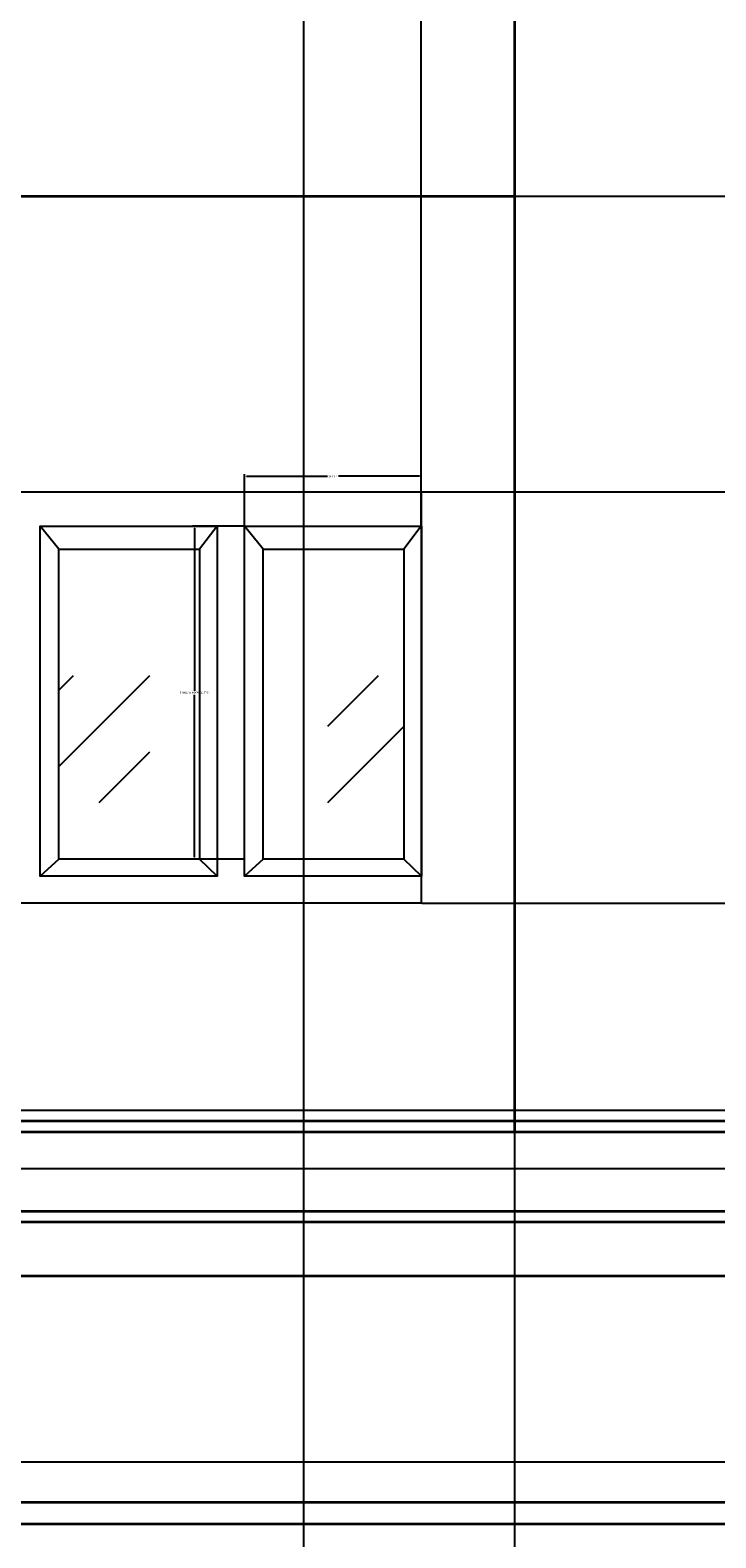
# Model space of a CAD drawing. Units: inches. Extents: x 93 to 565, y 123 to 656.
# Tile 10 of 18: x 393 to 456, y 324 to 463. Entities that reach past the tile are written whole.
import ezdxf

# ---------------------------------------------------------------- set-up
doc = ezdxf.new("R2010")
doc.units = ezdxf.units.IN
doc.header["$MEASUREMENT"] = 0
for name, color, linetype, lineweight in [('A-ANNO-DIMS', 2, 'Continuous', 18), ('A-ELEV', 7, 'Continuous', 35), ('A-GLAZ', 4, 'Continuous', 25)]:
    doc.layers.add(name, color=color, linetype=linetype, lineweight=lineweight)
doc.styles.get("Standard").update_dxf_attribs({"font": 'arial.ttf'})
doc.dimstyles.get("Standard").update_dxf_attribs({"dimtxt": 0.18, "dimasz": 0.18, "dimexe": 0.18, "dimexo": 0.0625, "dimgap": 0.09, "dimtad": 0, "dimtih": 1, "dimtoh": 1, "dimdec": 4, "dimzin": 0, "dimdsep": 46, "dimtxsty": 'Standard', "dimcen": 0.09, "dimadec": 0, "dimazin": 0, "dimtfac": 1, "dimtdec": 4, "dimtofl": 0, "dimtmove": 0, "dimatfit": 3, "dimfxl": 1, "dimtolj": 1, "dimtzin": 0, "dimarcsym": 0})

# ---------------------------------------------------------------- blocks, each defined once
blk = doc.blocks.new('WIN-CASEMENT-SMALL')
blk.add_lwpolyline([(1.71, 28.48), (0, 30.59), (16.23, 30.59), (14.61, 28.48)])
blk.add_lwpolyline([(1.71, 28.48), (14.61, 28.48), (14.61, 0), (1.71, 0)], close=True)
blk = doc.blocks.new('*D16')
at = {"layer": 'A-ANNO-DIMS', "color": 0, "lineweight": -2, "transparency": 16777216}
for p, q in [((412.34, 417.42), (407.63, 417.42)), ((407.81, 417.24), (407.81, 402.31)), ((407.81, 387.01), (407.81, 401.94)), ((412.34, 386.83), (407.63, 386.83))]:
    blk.add_line(p, q, dxfattribs=at)
at = {"layer": 'A-ANNO-DIMS', "color": 0, "transparency": 16777216}
for points in [[(407.78, 417.24), (407.84, 417.24), (407.81, 417.42)], [(407.78, 387.01), (407.84, 387.01), (407.81, 386.83)]]:
    blk.add_solid(points, dxfattribs=at)
at = {"layer": 'Defpoints', "color": 0, "transparency": 16777216}
for p in [(407.81, 417.42), (412.4, 417.42), (412.4, 386.83)]:
    blk.add_point(p, dxfattribs=at)
at = {"layer": 'A-ANNO-DIMS', "color": 0, "transparency": 16777216, "insert": (407.81, 402.13), "char_height": 0.18, "attachment_point": 5}
blk.add_mtext('\\A1;SMALL WINDOW 31 TYP.', dxfattribs=at)
blk = doc.blocks.new('*D17')
at = {"layer": 'A-ANNO-DIMS', "color": 0, "lineweight": -2, "transparency": 16777216}
for p, q in [((412.4, 417.49), (412.4, 422.19)), ((412.58, 422.01), (420, 422.01)), ((428.45, 422.01), (421.03, 422.01)), ((428.63, 417.49), (428.63, 422.19))]:
    blk.add_line(p, q, dxfattribs=at)
at = {"layer": 'A-ANNO-DIMS', "color": 0, "transparency": 16777216}
for points in [[(412.58, 422.04), (412.58, 421.98), (412.4, 422.01)], [(428.45, 422.04), (428.45, 421.98), (428.63, 422.01)]]:
    blk.add_solid(points, dxfattribs=at)
at = {"layer": 'Defpoints', "color": 0, "transparency": 16777216}
for p in [(428.63, 422.01), (412.4, 417.42), (428.63, 417.42)]:
    blk.add_point(p, dxfattribs=at)
at = {"layer": 'A-ANNO-DIMS', "color": 0, "transparency": 16777216, "insert": (420.51, 422.01), "char_height": 0.18, "attachment_point": 5}
blk.add_mtext('\\A1;16 TYP.', dxfattribs=at)
blk = doc.blocks.new('*D29')
at = {"layer": 'A-ANNO-DIMS', "color": 0, "lineweight": -2, "transparency": 16777216}
for p, q in [((437.19, 594.34), (437.19, 134)), ((295.69, 183.67), (295.69, 134)), ((295.87, 134.18), (366.05, 134.18)), ((437.01, 134.18), (366.82, 134.18))]:
    blk.add_line(p, q, dxfattribs=at)
at = {"layer": 'A-ANNO-DIMS', "color": 0, "transparency": 16777216}
for points in [[(295.87, 134.21), (295.87, 134.15), (295.69, 134.18)], [(437.01, 134.21), (437.01, 134.15), (437.19, 134.18)]]:
    blk.add_solid(points, dxfattribs=at)
at = {"layer": 'Defpoints', "color": 0, "transparency": 16777216}
for p in [(437.19, 594.4), (295.69, 183.73), (437.19, 134.18)]:
    blk.add_point(p, dxfattribs=at)
at = {"layer": 'A-ANNO-DIMS', "color": 0, "transparency": 16777216, "insert": (366.44, 134.18), "char_height": 0.18, "attachment_point": 5}
blk.add_mtext('\\A1;141.5', dxfattribs=at)
blk = doc.blocks.new('*D30')
at = {"layer": 'A-ANNO-DIMS', "color": 0, "lineweight": -2, "transparency": 16777216}
for p, q in [((437.19, 594.34), (437.19, 134)), ((539.08, 159.67), (539.08, 134)), ((437.37, 134.18), (487.75, 134.18)), ((538.9, 134.18), (488.52, 134.18))]:
    blk.add_line(p, q, dxfattribs=at)
at = {"layer": 'A-ANNO-DIMS', "color": 0, "transparency": 16777216}
for points in [[(437.37, 134.21), (437.37, 134.15), (437.19, 134.18)], [(538.9, 134.21), (538.9, 134.15), (539.08, 134.18)]]:
    blk.add_solid(points, dxfattribs=at)
at = {"layer": 'Defpoints', "color": 0, "transparency": 16777216}
for p in [(437.19, 594.4), (539.08, 159.73), (539.08, 134.18)]:
    blk.add_point(p, dxfattribs=at)
at = {"layer": 'A-ANNO-DIMS', "color": 0, "transparency": 16777216, "insert": (488.13, 134.18), "char_height": 0.18, "attachment_point": 5}
blk.add_mtext('\\A1;101.9', dxfattribs=at)
blk = doc.blocks.new('*D31')
at = {"layer": 'A-ANNO-DIMS', "color": 0, "lineweight": -2, "transparency": 16777216}
for p, q in [((417.87, 630.4), (564.81, 630.4)), ((564.63, 630.22), (564.63, 395.25)), ((564.63, 159.91), (564.63, 394.89)), ((119.14, 159.73), (564.81, 159.73))]:
    blk.add_line(p, q, dxfattribs=at)
at = {"layer": 'A-ANNO-DIMS', "color": 0, "transparency": 16777216}
for points in [[(564.6, 630.22), (564.66, 630.22), (564.63, 630.4)], [(564.6, 159.91), (564.66, 159.91), (564.63, 159.73)]]:
    blk.add_solid(points, dxfattribs=at)
at = {"layer": 'Defpoints', "color": 0, "transparency": 16777216}
for p in [(417.81, 630.4), (564.63, 630.4), (119.08, 159.73)]:
    blk.add_point(p, dxfattribs=at)
at = {"layer": 'A-ANNO-DIMS', "color": 0, "transparency": 16777216, "insert": (564.63, 395.07), "char_height": 0.18, "attachment_point": 5}
blk.add_mtext('\\A1;470.7', dxfattribs=at)
blk = doc.blocks.new('*D67')
at = {"layer": 'A-ANNO-DIMS', "color": 0, "lineweight": -2, "transparency": 16777216}
for p, q in [((331.87, 420.57), (564.81, 420.57)), ((564.63, 420.39), (564.63, 384.75)), ((564.63, 348.75), (564.63, 384.39)), ((331.87, 348.57), (564.81, 348.57))]:
    blk.add_line(p, q, dxfattribs=at)
at = {"layer": 'A-ANNO-DIMS', "color": 0, "transparency": 16777216}
for points in [[(564.6, 420.39), (564.66, 420.39), (564.63, 420.57)], [(564.6, 348.75), (564.66, 348.75), (564.63, 348.57)]]:
    blk.add_solid(points, dxfattribs=at)
at = {"layer": 'Defpoints', "color": 0, "transparency": 16777216}
for p in [(331.81, 420.57), (564.63, 420.57), (331.81, 348.57)]:
    blk.add_point(p, dxfattribs=at)
at = {"layer": 'A-ANNO-DIMS', "color": 0, "transparency": 16777216, "insert": (564.63, 384.57), "char_height": 0.18, "attachment_point": 5}
blk.add_mtext('\\A1;72', dxfattribs=at)
blk = doc.blocks.new('*D69')
at = {"layer": 'A-ANNO-DIMS', "color": 0, "lineweight": -2, "transparency": 16777216}
for p, q in [((355.46, 420.63), (355.46, 656.13)), ((355.64, 655.95), (391.65, 655.95)), ((428.44, 655.95), (392.43, 655.95)), ((428.62, 420.63), (428.62, 656.13))]:
    blk.add_line(p, q, dxfattribs=at)
at = {"layer": 'A-ANNO-DIMS', "color": 0, "transparency": 16777216}
for points in [[(355.64, 655.98), (355.64, 655.92), (355.46, 655.95)], [(428.44, 655.98), (428.44, 655.92), (428.62, 655.95)]]:
    blk.add_solid(points, dxfattribs=at)
at = {"layer": 'Defpoints', "color": 0, "transparency": 16777216}
for p in [(428.62, 655.95), (355.46, 420.57), (428.62, 420.57)]:
    blk.add_point(p, dxfattribs=at)
at = {"layer": 'A-ANNO-DIMS', "color": 0, "transparency": 16777216, "insert": (392.04, 655.95), "char_height": 0.18, "attachment_point": 5}
blk.add_mtext('\\A1;73.16', dxfattribs=at)
blk = doc.blocks.new('*D70')
at = {"layer": 'A-ANNO-DIMS', "color": 0, "lineweight": -2, "transparency": 16777216}
for p, q in [((428.68, 420.57), (564.81, 420.57)), ((564.63, 420.39), (564.63, 401.87)), ((564.63, 382.98), (564.63, 401.5)), ((428.68, 382.8), (564.81, 382.8))]:
    blk.add_line(p, q, dxfattribs=at)
at = {"layer": 'A-ANNO-DIMS', "color": 0, "transparency": 16777216}
for points in [[(564.6, 420.39), (564.66, 420.39), (564.63, 420.57)], [(564.6, 382.98), (564.66, 382.98), (564.63, 382.8)]]:
    blk.add_solid(points, dxfattribs=at)
at = {"layer": 'Defpoints', "color": 0, "transparency": 16777216}
for p in [(428.62, 420.57), (564.63, 420.57), (428.62, 382.8)]:
    blk.add_point(p, dxfattribs=at)
at = {"layer": 'A-ANNO-DIMS', "color": 0, "transparency": 16777216, "insert": (564.63, 401.68), "char_height": 0.18, "attachment_point": 5}
blk.add_mtext('\\A1;37.77', dxfattribs=at)
blk = doc.blocks.new('*D71')
at = {"layer": 'A-ANNO-DIMS', "color": 0, "lineweight": -2, "transparency": 16777216}
for p, q in [((428.68, 382.8), (564.81, 382.8)), ((564.63, 382.62), (564.63, 372.46)), ((564.63, 361.93), (564.63, 372.09)), ((437.25, 361.75), (564.81, 361.75))]:
    blk.add_line(p, q, dxfattribs=at)
at = {"layer": 'A-ANNO-DIMS', "color": 0, "transparency": 16777216}
for points in [[(564.6, 382.62), (564.66, 382.62), (564.63, 382.8)], [(564.6, 361.93), (564.66, 361.93), (564.63, 361.75)]]:
    blk.add_solid(points, dxfattribs=at)
at = {"layer": 'Defpoints', "color": 0, "transparency": 16777216}
for p in [(428.62, 382.8), (437.19, 361.75), (564.63, 361.75)]:
    blk.add_point(p, dxfattribs=at)
at = {"layer": 'A-ANNO-DIMS', "color": 0, "transparency": 16777216, "insert": (564.63, 372.27), "char_height": 0.18, "attachment_point": 5}
blk.add_mtext('\\A1;21.05', dxfattribs=at)
blk = doc.blocks.new('*D73')
at = {"layer": 'A-ANNO-DIMS', "color": 0, "lineweight": -2, "transparency": 16777216}
for p, q in [((437.25, 473.73), (564.81, 473.73)), ((564.63, 473.55), (564.63, 460.91)), ((564.63, 447.91), (564.63, 460.55)), ((437.25, 447.73), (564.81, 447.73))]:
    blk.add_line(p, q, dxfattribs=at)
at = {"layer": 'A-ANNO-DIMS', "color": 0, "transparency": 16777216}
for points in [[(564.6, 473.55), (564.66, 473.55), (564.63, 473.73)], [(564.6, 447.91), (564.66, 447.91), (564.63, 447.73)]]:
    blk.add_solid(points, dxfattribs=at)
at = {"layer": 'Defpoints', "color": 0, "transparency": 16777216}
for p in [(437.19, 473.73), (564.63, 473.73), (437.19, 447.73)]:
    blk.add_point(p, dxfattribs=at)
at = {"layer": 'A-ANNO-DIMS', "color": 0, "transparency": 16777216, "insert": (564.63, 460.73), "char_height": 0.18, "attachment_point": 5}
blk.add_mtext('\\A1;26', dxfattribs=at)
blk = doc.blocks.new('*D82')
at = {"layer": 'A-ANNO-DIMS', "color": 0, "lineweight": -2, "transparency": 16777216}
for p, q in [((437.19, 447.79), (437.19, 656.13)), ((437.37, 655.95), (446.83, 655.95)), ((457.21, 655.95), (447.76, 655.95)), ((457.39, 378.4), (457.39, 656.13))]:
    blk.add_line(p, q, dxfattribs=at)
at = {"layer": 'A-ANNO-DIMS', "color": 0, "transparency": 16777216}
for points in [[(437.37, 655.98), (437.37, 655.92), (437.19, 655.95)], [(457.21, 655.98), (457.21, 655.92), (457.39, 655.95)]]:
    blk.add_solid(points, dxfattribs=at)
at = {"layer": 'Defpoints', "color": 0, "transparency": 16777216}
for p in [(457.39, 655.95), (437.19, 447.73), (457.39, 378.34)]:
    blk.add_point(p, dxfattribs=at)
at = {"layer": 'A-ANNO-DIMS', "color": 0, "transparency": 16777216, "insert": (447.29, 655.95), "char_height": 0.18, "attachment_point": 5}
blk.add_mtext('\\A1;20.205', dxfattribs=at)
blk = doc.blocks.new('*D83')
at = {"layer": 'A-ANNO-DIMS', "color": 0, "lineweight": -2, "transparency": 16777216}
for p, q in [((457.46, 378.34), (564.81, 378.34)), ((564.63, 378.16), (564.63, 370.22)), ((564.63, 361.93), (564.63, 369.86)), ((437.25, 361.75), (564.81, 361.75))]:
    blk.add_line(p, q, dxfattribs=at)
at = {"layer": 'A-ANNO-DIMS', "color": 0, "transparency": 16777216}
for points in [[(564.6, 378.16), (564.66, 378.16), (564.63, 378.34)], [(564.6, 361.93), (564.66, 361.93), (564.63, 361.75)]]:
    blk.add_solid(points, dxfattribs=at)
at = {"layer": 'Defpoints', "color": 0, "transparency": 16777216}
for p in [(457.39, 378.34), (437.19, 361.75), (564.63, 361.75)]:
    blk.add_point(p, dxfattribs=at)
at = {"layer": 'A-ANNO-DIMS', "color": 0, "transparency": 16777216, "insert": (564.63, 370.04), "char_height": 0.18, "attachment_point": 5}
blk.add_mtext('\\A1;16.59', dxfattribs=at)
blk = doc.blocks.new('*D90')
at = {"layer": 'A-ANNO-DIMS', "color": 0, "lineweight": -2, "transparency": 16777216}
for p, q in [((417.81, 594.34), (417.81, 134)), ((437.19, 594.34), (437.19, 134)), ((417.99, 134.18), (427.11, 134.18)), ((437.01, 134.18), (427.88, 134.18))]:
    blk.add_line(p, q, dxfattribs=at)
at = {"layer": 'A-ANNO-DIMS', "color": 0, "transparency": 16777216}
for points in [[(417.99, 134.21), (417.99, 134.15), (417.81, 134.18)], [(437.01, 134.21), (437.01, 134.15), (437.19, 134.18)]]:
    blk.add_solid(points, dxfattribs=at)
at = {"layer": 'Defpoints', "color": 0, "transparency": 16777216}
for p in [(417.81, 594.4), (437.19, 594.4), (437.19, 134.18)]:
    blk.add_point(p, dxfattribs=at)
at = {"layer": 'A-ANNO-DIMS', "color": 0, "transparency": 16777216, "insert": (427.5, 134.18), "char_height": 0.18, "attachment_point": 5}
blk.add_mtext('\\A1;19.38', dxfattribs=at)
blk = doc.blocks.new('*D91')
at = {"layer": 'A-ANNO-DIMS', "color": 0, "lineweight": -2, "transparency": 16777216}
for p, q in [((499.73, 599.75), (499.73, 134)), ((437.19, 594.34), (437.19, 134)), ((437.37, 134.18), (468.07, 134.18)), ((499.55, 134.18), (468.85, 134.18))]:
    blk.add_line(p, q, dxfattribs=at)
at = {"layer": 'A-ANNO-DIMS', "color": 0, "transparency": 16777216}
for points in [[(437.37, 134.21), (437.37, 134.15), (437.19, 134.18)], [(499.55, 134.21), (499.55, 134.15), (499.73, 134.18)]]:
    blk.add_solid(points, dxfattribs=at)
at = {"layer": 'Defpoints', "color": 0, "transparency": 16777216}
for p in [(499.73, 599.82), (437.19, 594.4), (499.73, 134.18)]:
    blk.add_point(p, dxfattribs=at)
at = {"layer": 'A-ANNO-DIMS', "color": 0, "transparency": 16777216, "insert": (468.46, 134.18), "char_height": 0.18, "attachment_point": 5}
blk.add_mtext('\\A1;62.54', dxfattribs=at)
blk = doc.blocks.new('*D108')
at = {"layer": 'A-ANNO-DIMS', "color": 0, "lineweight": -2, "transparency": 16777216}
for p, q in [((437.19, 594.34), (437.19, 134)), ((295.69, 183.67), (295.69, 134)), ((295.87, 134.18), (365.93, 134.18)), ((437.01, 134.18), (366.95, 134.18))]:
    blk.add_line(p, q, dxfattribs=at)
at = {"layer": 'A-ANNO-DIMS', "color": 0, "transparency": 16777216}
for points in [[(295.87, 134.21), (295.87, 134.15), (295.69, 134.18)], [(437.01, 134.21), (437.01, 134.15), (437.19, 134.18)]]:
    blk.add_solid(points, dxfattribs=at)
at = {"layer": 'Defpoints', "color": 0, "transparency": 16777216}
for p in [(437.19, 594.4), (295.69, 183.73), (437.19, 134.18)]:
    blk.add_point(p, dxfattribs=at)
at = {"layer": 'A-ANNO-DIMS', "color": 0, "transparency": 16777216, "insert": (366.44, 134.18), "char_height": 0.18, "attachment_point": 5}
blk.add_mtext('\\A1;141.501', dxfattribs=at)
blk = doc.blocks.new('*D109')
at = {"layer": 'A-ANNO-DIMS', "color": 0, "lineweight": -2, "transparency": 16777216}
for p, q in [((437.19, 594.34), (437.19, 134)), ((539.08, 159.67), (539.08, 134)), ((437.37, 134.18), (487.63, 134.18)), ((538.9, 134.18), (488.64, 134.18))]:
    blk.add_line(p, q, dxfattribs=at)
at = {"layer": 'A-ANNO-DIMS', "color": 0, "transparency": 16777216}
for points in [[(437.37, 134.21), (437.37, 134.15), (437.19, 134.18)], [(538.9, 134.21), (538.9, 134.15), (539.08, 134.18)]]:
    blk.add_solid(points, dxfattribs=at)
at = {"layer": 'Defpoints', "color": 0, "transparency": 16777216}
for p in [(437.19, 594.4), (539.08, 159.73), (539.08, 134.18)]:
    blk.add_point(p, dxfattribs=at)
at = {"layer": 'A-ANNO-DIMS', "color": 0, "transparency": 16777216, "insert": (488.13, 134.18), "char_height": 0.18, "attachment_point": 5}
blk.add_mtext('\\A1;101.891', dxfattribs=at)
blk = doc.blocks.new('*D110')
at = {"layer": 'A-ANNO-DIMS', "color": 0, "lineweight": -2, "transparency": 16777216}
for p, q in [((417.87, 630.4), (564.81, 630.4)), ((564.63, 630.22), (564.63, 395.25)), ((564.63, 159.91), (564.63, 394.89)), ((119.14, 159.73), (564.81, 159.73))]:
    blk.add_line(p, q, dxfattribs=at)
at = {"layer": 'A-ANNO-DIMS', "color": 0, "transparency": 16777216}
for points in [[(564.6, 630.22), (564.66, 630.22), (564.63, 630.4)], [(564.6, 159.91), (564.66, 159.91), (564.63, 159.73)]]:
    blk.add_solid(points, dxfattribs=at)
at = {"layer": 'Defpoints', "color": 0, "transparency": 16777216}
for p in [(417.81, 630.4), (564.63, 630.4), (119.08, 159.73)]:
    blk.add_point(p, dxfattribs=at)
at = {"layer": 'A-ANNO-DIMS', "color": 0, "transparency": 16777216, "insert": (564.63, 395.07), "char_height": 0.18, "attachment_point": 5}
blk.add_mtext('\\A1;470.673', dxfattribs=at)
blk = doc.blocks.new('*D146')
at = {"layer": 'A-ANNO-DIMS', "color": 0, "lineweight": -2, "transparency": 16777216}
for p, q in [((331.87, 420.57), (564.81, 420.57)), ((564.63, 420.39), (564.63, 384.75)), ((564.63, 348.75), (564.63, 384.39)), ((331.87, 348.57), (564.81, 348.57))]:
    blk.add_line(p, q, dxfattribs=at)
at = {"layer": 'A-ANNO-DIMS', "color": 0, "transparency": 16777216}
for points in [[(564.6, 420.39), (564.66, 420.39), (564.63, 420.57)], [(564.6, 348.75), (564.66, 348.75), (564.63, 348.57)]]:
    blk.add_solid(points, dxfattribs=at)
at = {"layer": 'Defpoints', "color": 0, "transparency": 16777216}
for p in [(331.81, 420.57), (564.63, 420.57), (331.81, 348.57)]:
    blk.add_point(p, dxfattribs=at)
at = {"layer": 'A-ANNO-DIMS', "color": 0, "transparency": 16777216, "insert": (564.63, 384.57), "char_height": 0.18, "attachment_point": 5}
blk.add_mtext('\\A1;72.000', dxfattribs=at)
blk = doc.blocks.new('*D148')
at = {"layer": 'A-ANNO-DIMS', "color": 0, "lineweight": -2, "transparency": 16777216}
for p, q in [((355.46, 420.63), (355.46, 656.13)), ((355.64, 655.95), (391.58, 655.95)), ((428.44, 655.95), (392.5, 655.95)), ((428.62, 420.63), (428.62, 656.13))]:
    blk.add_line(p, q, dxfattribs=at)
at = {"layer": 'A-ANNO-DIMS', "color": 0, "transparency": 16777216}
for points in [[(355.64, 655.98), (355.64, 655.92), (355.46, 655.95)], [(428.44, 655.98), (428.44, 655.92), (428.62, 655.95)]]:
    blk.add_solid(points, dxfattribs=at)
at = {"layer": 'Defpoints', "color": 0, "transparency": 16777216}
for p in [(428.62, 655.95), (355.46, 420.57), (428.62, 420.57)]:
    blk.add_point(p, dxfattribs=at)
at = {"layer": 'A-ANNO-DIMS', "color": 0, "transparency": 16777216, "insert": (392.04, 655.95), "char_height": 0.18, "attachment_point": 5}
blk.add_mtext('\\A1;73.156', dxfattribs=at)
blk = doc.blocks.new('*D149')
at = {"layer": 'A-ANNO-DIMS', "color": 0, "lineweight": -2, "transparency": 16777216}
for p, q in [((428.68, 420.57), (564.81, 420.57)), ((564.63, 420.39), (564.63, 401.87)), ((564.63, 382.98), (564.63, 401.5)), ((428.68, 382.8), (564.81, 382.8))]:
    blk.add_line(p, q, dxfattribs=at)
at = {"layer": 'A-ANNO-DIMS', "color": 0, "transparency": 16777216}
for points in [[(564.6, 420.39), (564.66, 420.39), (564.63, 420.57)], [(564.6, 382.98), (564.66, 382.98), (564.63, 382.8)]]:
    blk.add_solid(points, dxfattribs=at)
at = {"layer": 'Defpoints', "color": 0, "transparency": 16777216}
for p in [(428.62, 420.57), (564.63, 420.57), (428.62, 382.8)]:
    blk.add_point(p, dxfattribs=at)
at = {"layer": 'A-ANNO-DIMS', "color": 0, "transparency": 16777216, "insert": (564.63, 401.68), "char_height": 0.18, "attachment_point": 5}
blk.add_mtext('\\A1;37.768', dxfattribs=at)
blk = doc.blocks.new('*D150')
at = {"layer": 'A-ANNO-DIMS', "color": 0, "lineweight": -2, "transparency": 16777216}
for p, q in [((428.68, 382.8), (564.81, 382.8)), ((564.63, 382.62), (564.63, 372.46)), ((564.63, 361.93), (564.63, 372.09)), ((437.25, 361.75), (564.81, 361.75))]:
    blk.add_line(p, q, dxfattribs=at)
at = {"layer": 'A-ANNO-DIMS', "color": 0, "transparency": 16777216}
for points in [[(564.6, 382.62), (564.66, 382.62), (564.63, 382.8)], [(564.6, 361.93), (564.66, 361.93), (564.63, 361.75)]]:
    blk.add_solid(points, dxfattribs=at)
at = {"layer": 'Defpoints', "color": 0, "transparency": 16777216}
for p in [(428.62, 382.8), (437.19, 361.75), (564.63, 361.75)]:
    blk.add_point(p, dxfattribs=at)
at = {"layer": 'A-ANNO-DIMS', "color": 0, "transparency": 16777216, "insert": (564.63, 372.27), "char_height": 0.18, "attachment_point": 5}
blk.add_mtext('\\A1;21.052', dxfattribs=at)
blk = doc.blocks.new('*D152')
at = {"layer": 'A-ANNO-DIMS', "color": 0, "lineweight": -2, "transparency": 16777216}
for p, q in [((437.25, 473.73), (564.81, 473.73)), ((564.63, 473.55), (564.63, 460.91)), ((564.63, 447.91), (564.63, 460.55)), ((437.25, 447.73), (564.81, 447.73))]:
    blk.add_line(p, q, dxfattribs=at)
at = {"layer": 'A-ANNO-DIMS', "color": 0, "transparency": 16777216}
for points in [[(564.6, 473.55), (564.66, 473.55), (564.63, 473.73)], [(564.6, 447.91), (564.66, 447.91), (564.63, 447.73)]]:
    blk.add_solid(points, dxfattribs=at)
at = {"layer": 'Defpoints', "color": 0, "transparency": 16777216}
for p in [(437.19, 473.73), (564.63, 473.73), (437.19, 447.73)]:
    blk.add_point(p, dxfattribs=at)
at = {"layer": 'A-ANNO-DIMS', "color": 0, "transparency": 16777216, "insert": (564.63, 460.73), "char_height": 0.18, "attachment_point": 5}
blk.add_mtext('\\A1;26.000', dxfattribs=at)
blk = doc.blocks.new('*D161')
at = {"layer": 'A-ANNO-DIMS', "color": 0, "lineweight": -2, "transparency": 16777216}
for p, q in [((437.19, 447.79), (437.19, 656.13)), ((437.37, 655.95), (446.83, 655.95)), ((457.21, 655.95), (447.76, 655.95)), ((457.39, 378.4), (457.39, 656.13))]:
    blk.add_line(p, q, dxfattribs=at)
at = {"layer": 'A-ANNO-DIMS', "color": 0, "transparency": 16777216}
for points in [[(437.37, 655.98), (437.37, 655.92), (437.19, 655.95)], [(457.21, 655.98), (457.21, 655.92), (457.39, 655.95)]]:
    blk.add_solid(points, dxfattribs=at)
at = {"layer": 'Defpoints', "color": 0, "transparency": 16777216}
for p in [(457.39, 655.95), (437.19, 447.73), (457.39, 378.34)]:
    blk.add_point(p, dxfattribs=at)
at = {"layer": 'A-ANNO-DIMS', "color": 0, "transparency": 16777216, "insert": (447.29, 655.95), "char_height": 0.18, "attachment_point": 5}
blk.add_mtext('\\A1;20.205', dxfattribs=at)
blk = doc.blocks.new('*D162')
at = {"layer": 'A-ANNO-DIMS', "color": 0, "lineweight": -2, "transparency": 16777216}
for p, q in [((457.46, 378.34), (564.81, 378.34)), ((564.63, 378.16), (564.63, 370.22)), ((564.63, 361.93), (564.63, 369.86)), ((437.25, 361.75), (564.81, 361.75))]:
    blk.add_line(p, q, dxfattribs=at)
at = {"layer": 'A-ANNO-DIMS', "color": 0, "transparency": 16777216}
for points in [[(564.6, 378.16), (564.66, 378.16), (564.63, 378.34)], [(564.6, 361.93), (564.66, 361.93), (564.63, 361.75)]]:
    blk.add_solid(points, dxfattribs=at)
at = {"layer": 'Defpoints', "color": 0, "transparency": 16777216}
for p in [(457.39, 378.34), (437.19, 361.75), (564.63, 361.75)]:
    blk.add_point(p, dxfattribs=at)
at = {"layer": 'A-ANNO-DIMS', "color": 0, "transparency": 16777216, "insert": (564.63, 370.04), "char_height": 0.18, "attachment_point": 5}
blk.add_mtext('\\A1;16.590', dxfattribs=at)
blk = doc.blocks.new('*D169')
at = {"layer": 'A-ANNO-DIMS', "color": 0, "lineweight": -2, "transparency": 16777216}
for p, q in [((417.81, 594.34), (417.81, 134)), ((437.19, 594.34), (437.19, 134)), ((417.99, 134.18), (427.04, 134.18)), ((437.01, 134.18), (427.95, 134.18))]:
    blk.add_line(p, q, dxfattribs=at)
at = {"layer": 'A-ANNO-DIMS', "color": 0, "transparency": 16777216}
for points in [[(417.99, 134.21), (417.99, 134.15), (417.81, 134.18)], [(437.01, 134.21), (437.01, 134.15), (437.19, 134.18)]]:
    blk.add_solid(points, dxfattribs=at)
at = {"layer": 'Defpoints', "color": 0, "transparency": 16777216}
for p in [(417.81, 594.4), (437.19, 594.4), (437.19, 134.18)]:
    blk.add_point(p, dxfattribs=at)
at = {"layer": 'A-ANNO-DIMS', "color": 0, "transparency": 16777216, "insert": (427.5, 134.18), "char_height": 0.18, "attachment_point": 5}
blk.add_mtext('\\A1;19.379', dxfattribs=at)
blk = doc.blocks.new('*D170')
at = {"layer": 'A-ANNO-DIMS', "color": 0, "lineweight": -2, "transparency": 16777216}
for p, q in [((499.73, 599.75), (499.73, 134)), ((437.19, 594.34), (437.19, 134)), ((437.37, 134.18), (468.01, 134.18)), ((499.55, 134.18), (468.91, 134.18))]:
    blk.add_line(p, q, dxfattribs=at)
at = {"layer": 'A-ANNO-DIMS', "color": 0, "transparency": 16777216}
for points in [[(437.37, 134.21), (437.37, 134.15), (437.19, 134.18)], [(499.55, 134.21), (499.55, 134.15), (499.73, 134.18)]]:
    blk.add_solid(points, dxfattribs=at)
at = {"layer": 'Defpoints', "color": 0, "transparency": 16777216}
for p in [(499.73, 599.82), (437.19, 594.4), (499.73, 134.18)]:
    blk.add_point(p, dxfattribs=at)
at = {"layer": 'A-ANNO-DIMS', "color": 0, "transparency": 16777216, "insert": (468.46, 134.18), "char_height": 0.18, "attachment_point": 5}
blk.add_mtext('\\A1;62.541', dxfattribs=at)
blk = doc.blocks.new('*D190')
at = {"layer": 'A-ANNO-DIMS', "color": 0, "lineweight": -2, "transparency": 16777216}
for p, q in [((514.58, 348.55), (93.35, 348.55)), ((93.53, 348.37), (93.53, 338.33)), ((93.53, 327.91), (93.53, 337.96)), ((539.02, 327.73), (93.35, 327.73))]:
    blk.add_line(p, q, dxfattribs=at)
at = {"layer": 'A-ANNO-DIMS', "color": 0, "transparency": 16777216}
for points in [[(93.5, 348.37), (93.56, 348.37), (93.53, 348.55)], [(93.5, 327.91), (93.56, 327.91), (93.53, 327.73)]]:
    blk.add_solid(points, dxfattribs=at)
at = {"layer": 'Defpoints', "color": 0, "transparency": 16777216}
for p in [(93.53, 348.55), (514.64, 348.55), (539.08, 327.73)]:
    blk.add_point(p, dxfattribs=at)
at = {"layer": 'A-ANNO-DIMS', "color": 0, "transparency": 16777216, "insert": (93.53, 338.14), "char_height": 0.18, "attachment_point": 5}
blk.add_mtext('\\A1;20.822', dxfattribs=at)
blk = doc.blocks.new('*D191')
at = {"layer": 'A-ANNO-DIMS', "color": 0, "lineweight": -2, "transparency": 16777216}
for p, q in [((514.58, 353.47), (93.35, 353.47)), ((93.53, 353.29), (93.53, 351.2)), ((93.53, 348.73), (93.53, 350.83)), ((514.58, 348.55), (93.35, 348.55))]:
    blk.add_line(p, q, dxfattribs=at)
at = {"layer": 'A-ANNO-DIMS', "color": 0, "transparency": 16777216}
for points in [[(93.5, 353.29), (93.56, 353.29), (93.53, 353.47)], [(93.5, 348.73), (93.56, 348.73), (93.53, 348.55)]]:
    blk.add_solid(points, dxfattribs=at)
at = {"layer": 'Defpoints', "color": 0, "transparency": 16777216}
for p in [(93.53, 353.47), (514.64, 353.47), (514.64, 348.55)]:
    blk.add_point(p, dxfattribs=at)
at = {"layer": 'A-ANNO-DIMS', "color": 0, "transparency": 16777216, "insert": (93.53, 351.01), "char_height": 0.18, "attachment_point": 5}
blk.add_mtext('\\A1;4.918', dxfattribs=at)
blk = doc.blocks.new('*D192')
at = {"layer": 'A-ANNO-DIMS', "color": 0, "lineweight": -2, "transparency": 16777216}
for p, q in [((514.58, 354.47), (93.35, 354.47)), ((514.58, 353.47), (93.35, 353.47)), ((93.53, 354.29), (93.53, 354.15)), ((93.53, 353.65), (93.53, 353.79))]:
    blk.add_line(p, q, dxfattribs=at)
at = {"layer": 'A-ANNO-DIMS', "color": 0, "transparency": 16777216}
for points in [[(93.5, 354.29), (93.56, 354.29), (93.53, 354.47)], [(93.5, 353.65), (93.56, 353.65), (93.53, 353.47)]]:
    blk.add_solid(points, dxfattribs=at)
at = {"layer": 'Defpoints', "color": 0, "transparency": 16777216}
for p in [(93.53, 354.47), (514.64, 354.47), (514.64, 353.47)]:
    blk.add_point(p, dxfattribs=at)
at = {"layer": 'A-ANNO-DIMS', "color": 0, "transparency": 16777216, "insert": (93.53, 353.97), "char_height": 0.18, "attachment_point": 5}
blk.add_mtext('\\A1;1.000', dxfattribs=at)
blk = doc.blocks.new('*D193')
at = {"layer": 'A-ANNO-DIMS', "color": 0, "lineweight": -2, "transparency": 16777216}
for p, q in [((514.58, 358.37), (93.35, 358.37)), ((93.53, 358.19), (93.53, 356.61)), ((93.53, 354.65), (93.53, 356.24)), ((514.58, 354.47), (93.35, 354.47))]:
    blk.add_line(p, q, dxfattribs=at)
at = {"layer": 'A-ANNO-DIMS', "color": 0, "transparency": 16777216}
for points in [[(93.5, 358.19), (93.56, 358.19), (93.53, 358.37)], [(93.5, 354.65), (93.56, 354.65), (93.53, 354.47)]]:
    blk.add_solid(points, dxfattribs=at)
at = {"layer": 'Defpoints', "color": 0, "transparency": 16777216}
for p in [(93.53, 358.37), (514.64, 358.37), (514.64, 354.47)]:
    blk.add_point(p, dxfattribs=at)
at = {"layer": 'A-ANNO-DIMS', "color": 0, "transparency": 16777216, "insert": (93.53, 356.42), "char_height": 0.18, "attachment_point": 5}
blk.add_mtext('\\A1;3.901', dxfattribs=at)
blk = doc.blocks.new('*D194')
at = {"layer": 'A-ANNO-DIMS', "color": 0, "lineweight": -2, "transparency": 16777216}
for p, q in [((524.92, 361.75), (93.35, 361.75)), ((93.53, 361.57), (93.53, 360.24)), ((93.53, 358.55), (93.53, 359.88)), ((514.58, 358.37), (93.35, 358.37))]:
    blk.add_line(p, q, dxfattribs=at)
at = {"layer": 'A-ANNO-DIMS', "color": 0, "transparency": 16777216}
for points in [[(93.5, 361.57), (93.56, 361.57), (93.53, 361.75)], [(93.5, 358.55), (93.56, 358.55), (93.53, 358.37)]]:
    blk.add_solid(points, dxfattribs=at)
at = {"layer": 'Defpoints', "color": 0, "transparency": 16777216}
for p in [(93.53, 361.75), (524.99, 361.75), (514.64, 358.37)]:
    blk.add_point(p, dxfattribs=at)
at = {"layer": 'A-ANNO-DIMS', "color": 0, "transparency": 16777216, "insert": (93.53, 360.06), "char_height": 0.18, "attachment_point": 5}
blk.add_mtext('\\A1;3.374', dxfattribs=at)
blk = doc.blocks.new('*D195')
at = {"layer": 'A-ANNO-DIMS', "color": 0, "lineweight": -2, "transparency": 16777216}
for p, q in [((524.92, 362.75), (93.35, 362.75)), ((524.92, 361.75), (93.35, 361.75)), ((93.53, 362.57), (93.53, 362.43)), ((93.53, 361.93), (93.53, 362.07))]:
    blk.add_line(p, q, dxfattribs=at)
at = {"layer": 'A-ANNO-DIMS', "color": 0, "transparency": 16777216}
for points in [[(93.5, 362.57), (93.56, 362.57), (93.53, 362.75)], [(93.5, 361.93), (93.56, 361.93), (93.53, 361.75)]]:
    blk.add_solid(points, dxfattribs=at)
at = {"layer": 'Defpoints', "color": 0, "transparency": 16777216}
for p in [(93.53, 362.75), (524.99, 362.75), (524.99, 361.75)]:
    blk.add_point(p, dxfattribs=at)
at = {"layer": 'A-ANNO-DIMS', "color": 0, "transparency": 16777216, "insert": (93.53, 362.25), "char_height": 0.18, "attachment_point": 5}
blk.add_mtext('\\A1;1.000', dxfattribs=at)
blk = doc.blocks.new('*D196')
at = {"layer": 'A-ANNO-DIMS', "color": 0, "lineweight": -2, "transparency": 16777216}
for p, q in [((524.92, 363.73), (93.35, 363.73)), ((93.53, 363.55), (93.53, 363.42)), ((93.53, 362.93), (93.53, 363.06)), ((524.92, 362.75), (93.35, 362.75))]:
    blk.add_line(p, q, dxfattribs=at)
at = {"layer": 'A-ANNO-DIMS', "color": 0, "transparency": 16777216}
for points in [[(93.5, 363.55), (93.56, 363.55), (93.53, 363.73)], [(93.5, 362.93), (93.56, 362.93), (93.53, 362.75)]]:
    blk.add_solid(points, dxfattribs=at)
at = {"layer": 'Defpoints', "color": 0, "transparency": 16777216}
for p in [(93.53, 363.73), (524.99, 363.73), (524.99, 362.75)]:
    blk.add_point(p, dxfattribs=at)
at = {"layer": 'A-ANNO-DIMS', "color": 0, "transparency": 16777216, "insert": (93.53, 363.24), "char_height": 0.18, "attachment_point": 5}
blk.add_mtext('\\A1;0.985', dxfattribs=at)
blk = doc.blocks.new('*D198')
at = {"layer": 'A-ANNO-DIMS', "color": 0, "lineweight": -2, "transparency": 16777216}
for p, q in [((515.95, 331.43), (93.35, 331.43)), ((93.53, 331.25), (93.53, 329.76)), ((93.53, 327.91), (93.53, 329.4)), ((539.02, 327.73), (93.35, 327.73))]:
    blk.add_line(p, q, dxfattribs=at)
at = {"layer": 'A-ANNO-DIMS', "color": 0, "transparency": 16777216}
for points in [[(93.5, 331.25), (93.56, 331.25), (93.53, 331.43)], [(93.5, 327.91), (93.56, 327.91), (93.53, 327.73)]]:
    blk.add_solid(points, dxfattribs=at)
at = {"layer": 'Defpoints', "color": 0, "transparency": 16777216}
for p in [(93.53, 331.43), (516.01, 331.43), (539.08, 327.73)]:
    blk.add_point(p, dxfattribs=at)
at = {"layer": 'A-ANNO-DIMS', "color": 0, "transparency": 16777216, "insert": (93.53, 329.58), "char_height": 0.18, "attachment_point": 5}
blk.add_mtext('\\A1;3.701', dxfattribs=at)

msp = doc.modelspace()

# ---------------------------------------------------------------- hatches: boundary and pattern name
at = {"layer": 'A-GLAZ'}
h = msp.add_hatch(dxfattribs=at)
h.set_pattern_fill('GOST_GLASS', color=256, scale=3.3)
h.set_pattern_definition([(45, (0, 0), (28.0014, 0), [16.5, -23.1]), (45, (7, 0), (28.0014, 0), [6.6, -33]), (45, (0, 7), (28.0014, 0), [6.6, -33])])
h.paths.add_polyline_path([(332.6288, 267.5414), (312.4161, 267.5414), (312.4161, 222.941), (332.6288, 222.941)])
h.paths.add_polyline_path([(370.0743, 415.3107), (357.167, 415.3107), (357.167, 386.8299), (370.0743, 386.8299)])
h.paths.add_polyline_path([(390.168, 415.3107), (377.2607, 415.3107), (377.2607, 386.8299), (390.168, 386.8299)])
h.paths.add_polyline_path([(408.2592, 415.3107), (395.3518, 415.3107), (395.3518, 386.8299), (408.2592, 386.8299)])
h.paths.add_polyline_path([(427.0129, 415.3107), (414.1056, 415.3107), (414.1056, 386.8299), (427.0129, 386.8299)])

# ---------------------------------------------------------------- linework, layer by layer
at = {"layer": 'A-ELEV'}
for p, q in [((437.1885, 507.7323), (437.1885, 447.7323)), ((295.6874, 447.7323), (437.1885, 447.7323)), ((437.1885, 447.7323), (437.1885, 361.7477)), ((524.9864, 362.7477), (295.6874, 362.7477)), ((524.9864, 361.7477), (295.6874, 361.7477)), ((514.6424, 354.4729), (295.6874, 354.4729)), ((514.6424, 353.4729), (295.6874, 353.4729)), ((295.6874, 348.5546), (514.6424, 348.5546)), ((539.0794, 327.7323), (295.6874, 327.7323)), ((539.0794, 325.7323), (295.6874, 325.7323))]:
    msp.add_line(p, q, dxfattribs=at)
at = {"layer": 'A-GLAZ'}
for p, q in [((409.8769, 385.2642), (393.6451, 385.2642)), ((428.6307, 385.2642), (412.3989, 385.2642))]:
    msp.add_line(p, q, dxfattribs=at)
msp.add_lwpolyline([(355.4603, 420.5674), (428.6158, 420.5674), (428.6158, 382.7996), (355.4603, 382.7996)], close=True, dxfattribs=at)
for points in [[(395.3518, 386.8299), (393.6451, 385.2642), (393.6451, 417.4228)], [(409.8769, 417.4228), (409.8769, 385.2642), (408.2592, 386.8299)], [(414.1056, 386.8299), (412.3989, 385.2642), (412.3989, 417.4228)], [(428.6307, 417.4228), (428.6307, 385.2642), (427.0129, 386.8299)]]:
    msp.add_lwpolyline(points, dxfattribs=at)

# ---------------------------------------------------------------- block references
for p in [(393.6448, 386.83), (412.3986, 386.83)]:
    msp.add_blockref('WIN-CASEMENT-SMALL', p, dxfattribs=at)

# ---------------------------------------------------------------- dimensions: what is measured, and where the dimension line sits
at = {"layer": 'A-ANNO-DIMS'}
for base, p1, p2, override, picture, middle in [((428.6158, 655.9548), (355.4603, 420.5674), (428.6158, 420.5674), {"dimdec": 2, "dimlfac": 1, "dimrnd": 0, "dimzin": 0, "dimdsep": 46, "dimlunit": 2}, '*D69', (392.038, 655.9548)), ((428.615792, 655.954775), (355.460288, 420.567351), (428.615792, 420.567351), {"dimdec": 3, "dimlfac": 1, "dimrnd": 0, "dimzin": 0, "dimdsep": 46, "dimlunit": 2}, '*D148', (392.03804, 655.954775)), ((457.3933, 655.9548), (437.1885, 447.7323), (457.3933, 378.3372), {"dimdec": 3, "dimlfac": 1, "dimrnd": 0, "dimzin": 0, "dimdsep": 46, "dimlunit": 2}, '*D82', (447.2909, 655.9548)), ((457.3933, 655.9548), (437.1885, 447.7323), (457.3933, 378.3372), {"dimdec": 3, "dimlfac": 1, "dimrnd": 0, "dimzin": 0, "dimdsep": 46, "dimlunit": 2}, '*D161', (447.2909, 655.9548)), ((499.7291, 134.1823), (437.1885, 594.4048), (499.7291, 599.8171), {"dimdec": 2, "dimlfac": 1, "dimrnd": 0, "dimzin": 0, "dimdsep": 46, "dimlunit": 2}, '*D91', (468.4588, 134.1823)), ((499.7291, 134.1823), (437.1885, 594.4048), (499.7291, 599.8171), {"dimdec": 3, "dimlfac": 1, "dimrnd": 0, "dimzin": 0, "dimdsep": 46, "dimlunit": 2}, '*D170', (468.4588, 134.1823)), ((437.1885, 134.1823), (295.6874, 183.7323), (437.1885, 594.4048), {"dimdec": 1, "dimlfac": 1, "dimrnd": 0, "dimzin": 0, "dimdsep": 46, "dimlunit": 2}, '*D29', (366.438, 134.1823)), ((437.1885, 134.1823), (295.6874, 183.7323), (437.1885, 594.4048), {"dimdec": 3, "dimlfac": 1, "dimrnd": 0, "dimzin": 0, "dimdsep": 46, "dimlunit": 2}, '*D108', (366.438, 134.1823)), ((437.1885, 134.1823), (417.8097, 594.4048), (437.1885, 594.4048), {"dimdec": 2, "dimlfac": 1, "dimrnd": 0, "dimzin": 0, "dimdsep": 46, "dimlunit": 2}, '*D90', (427.4991, 134.1823)), ((437.1885, 134.1823), (417.8097, 594.4048), (437.1885, 594.4048), {"dimdec": 3, "dimlfac": 1, "dimrnd": 0, "dimzin": 0, "dimdsep": 46, "dimlunit": 2}, '*D169', (427.4991, 134.1823)), ((539.0794, 134.1823), (437.1885, 594.4048), (539.0794, 159.7323), {"dimdec": 1, "dimlfac": 1, "dimrnd": 0, "dimzin": 0, "dimdsep": 46, "dimlunit": 2}, '*D30', (488.1339, 134.1823)), ((539.0794, 134.1823), (437.1885, 594.4048), (539.0794, 159.7323), {"dimdec": 3, "dimlfac": 1, "dimrnd": 0, "dimzin": 0, "dimdsep": 46, "dimlunit": 2}, '*D109', (488.1339, 134.1823))]:
    dim = msp.add_linear_dim(base=base, p1=p1, p2=p2, dimstyle='Standard', override=override, dxfattribs=at)
    dim.commit()
    dim.dimension.update_dxf_attribs({"geometry": picture, "text_midpoint": middle})
for base, p1, p2, override, picture, middle in [((564.6294, 630.4048), (119.0794, 159.7323), (417.8097, 630.4048), {"dimdec": 1, "dimlfac": 1, "dimrnd": 0, "dimzin": 0, "dimdsep": 46, "dimlunit": 2}, '*D31', (564.6294, 395.0685)), ((564.62936, 630.40478), (119.07936, 159.73225), (417.80971, 630.40477), {"dimdec": 3, "dimlfac": 1, "dimrnd": 0, "dimzin": 0, "dimdsep": 46, "dimlunit": 2}, '*D110', (564.62936, 395.06851)), ((564.6294, 473.7323), (437.1885, 447.7323), (437.1885, 473.7323), {"dimdec": 0, "dimlfac": 1, "dimrnd": 0, "dimzin": 0, "dimdsep": 46, "dimlunit": 2}, '*D73', (564.6294, 460.7323)), ((564.6294, 473.7323), (437.1885, 447.7323), (437.1885, 473.7323), {"dimdec": 3, "dimlfac": 1, "dimrnd": 0, "dimzin": 0, "dimdsep": 46, "dimlunit": 2}, '*D152', (564.6294, 460.7323)), ((564.6294, 420.5674), (331.8112, 348.5674), (331.8112, 420.5674), {"dimdec": 0, "dimlfac": 1, "dimrnd": 0, "dimzin": 0, "dimdsep": 46, "dimlunit": 2}, '*D67', (564.6294, 384.5674)), ((564.6294, 420.5674), (331.8112, 348.5674), (331.8112, 420.5674), {"dimdec": 3, "dimlfac": 1, "dimrnd": 0, "dimzin": 0, "dimdsep": 46, "dimlunit": 2}, '*D146', (564.6294, 384.5674)), ((564.6294, 420.5674), (428.6158, 382.7996), (428.6158, 420.5674), {"dimdec": 2, "dimlfac": 1, "dimrnd": 0, "dimzin": 0, "dimdsep": 46, "dimlunit": 2}, '*D70', (564.6294, 401.6835)), ((564.6294, 420.5674), (428.6158, 382.7996), (428.6158, 420.5674), {"dimdec": 3, "dimlfac": 1, "dimrnd": 0, "dimzin": 0, "dimdsep": 46, "dimlunit": 2}, '*D149', (564.6294, 401.6835)), ((564.6294, 361.7477), (428.6158, 382.7996), (437.1885, 361.7477), {"dimdec": 2, "dimlfac": 1, "dimrnd": 0, "dimzin": 0, "dimdsep": 46, "dimlunit": 2}, '*D71', (564.6294, 372.2736)), ((564.6294, 361.7477), (428.6158, 382.7996), (437.1885, 361.7477), {"dimdec": 3, "dimlfac": 1, "dimrnd": 0, "dimzin": 0, "dimdsep": 46, "dimlunit": 2}, '*D150', (564.6294, 372.2736)), ((564.6294, 361.7477), (457.3933, 378.3372), (437.1885, 361.7477), {"dimdec": 2, "dimlfac": 1, "dimrnd": 0, "dimzin": 0, "dimdsep": 46, "dimlunit": 2}, '*D83', (564.6294, 370.0424)), ((564.62936, 361.74766), (457.3933, 378.33724), (437.18851, 361.74766), {"dimdec": 3, "dimlfac": 1, "dimrnd": 0, "dimzin": 0, "dimdsep": 46, "dimlunit": 2}, '*D162', (564.62936, 370.04245)), ((93.5294, 363.7323), (524.9864, 362.7477), (524.9864, 363.7323), {"dimdec": 3, "dimlfac": 1, "dimrnd": 0, "dimzin": 0, "dimdsep": 46, "dimlunit": 2}, '*D196', (93.5294, 363.24)), ((93.5294, 362.7477), (524.9864, 361.7477), (524.9864, 362.7477), {"dimdec": 3, "dimlfac": 1, "dimrnd": 0, "dimzin": 0, "dimdsep": 46, "dimlunit": 2}, '*D195', (93.5294, 362.2477)), ((93.5294, 361.7477), (514.6424, 358.3735), (524.9864, 361.7477), {"dimdec": 3, "dimlfac": 1, "dimrnd": 0, "dimzin": 0, "dimdsep": 46, "dimlunit": 2}, '*D194', (93.5294, 360.0606)), ((93.5294, 358.3735), (514.6424, 354.4729), (514.6424, 358.3735), {"dimdec": 3, "dimlfac": 1, "dimrnd": 0, "dimzin": 0, "dimdsep": 46, "dimlunit": 2}, '*D193', (93.5294, 356.4232)), ((93.5294, 354.4729), (514.6424, 353.4729), (514.6424, 354.4729), {"dimdec": 3, "dimlfac": 1, "dimrnd": 0, "dimzin": 0, "dimdsep": 46, "dimlunit": 2}, '*D192', (93.5294, 353.9729)), ((93.5294, 353.4729), (514.6424, 348.5546), (514.6424, 353.4729), {"dimdec": 3, "dimlfac": 1, "dimrnd": 0, "dimzin": 0, "dimdsep": 46, "dimlunit": 2}, '*D191', (93.5294, 351.0137)), ((93.5294, 348.5546), (539.0794, 327.7323), (514.6424, 348.5546), {"dimdec": 3, "dimlfac": 1, "dimrnd": 0, "dimzin": 0, "dimdsep": 46, "dimlunit": 2}, '*D190', (93.5294, 338.1434)), ((93.5294, 331.4335), (539.0794, 327.7323), (516.0099, 331.4335), {"dimdec": 3, "dimlfac": 1, "dimrnd": 0, "dimzin": 0, "dimdsep": 46, "dimlunit": 2}, '*D198', (93.5294, 329.5829))]:
    dim = msp.add_linear_dim(base=base, p1=p1, p2=p2, angle=90, dimstyle='Standard', override=override, dxfattribs=at)
    dim.commit()
    dim.dimension.update_dxf_attribs({"geometry": picture, "text_midpoint": middle})
dim = msp.add_linear_dim(base=(428.6307, 422.0117), p1=(412.3989, 417.4228), p2=(428.6307, 417.4228), text='<> TYP.', dimstyle='Standard', override={"dimdec": 0, "dimrnd": 0, "dimzin": 0, "dimlunit": 2}, dxfattribs=at)
dim.commit()
dim.dimension.update_dxf_attribs({"geometry": '*D17', "text_midpoint": (420.5148, 422.0117)})
dim = msp.add_linear_dim(base=(407.81, 417.4228), p1=(412.3989, 386.8299), p2=(412.3989, 417.4228), angle=90, text='SMALL WINDOW <> TYP.', dimstyle='Standard', override={"dimdec": 0, "dimrnd": 0, "dimzin": 0, "dimlunit": 2}, dxfattribs=at)
dim.commit()
dim.dimension.update_dxf_attribs({"geometry": '*D16', "text_midpoint": (407.81, 402.1263)})

doc.saveas('drawing.dxf')
